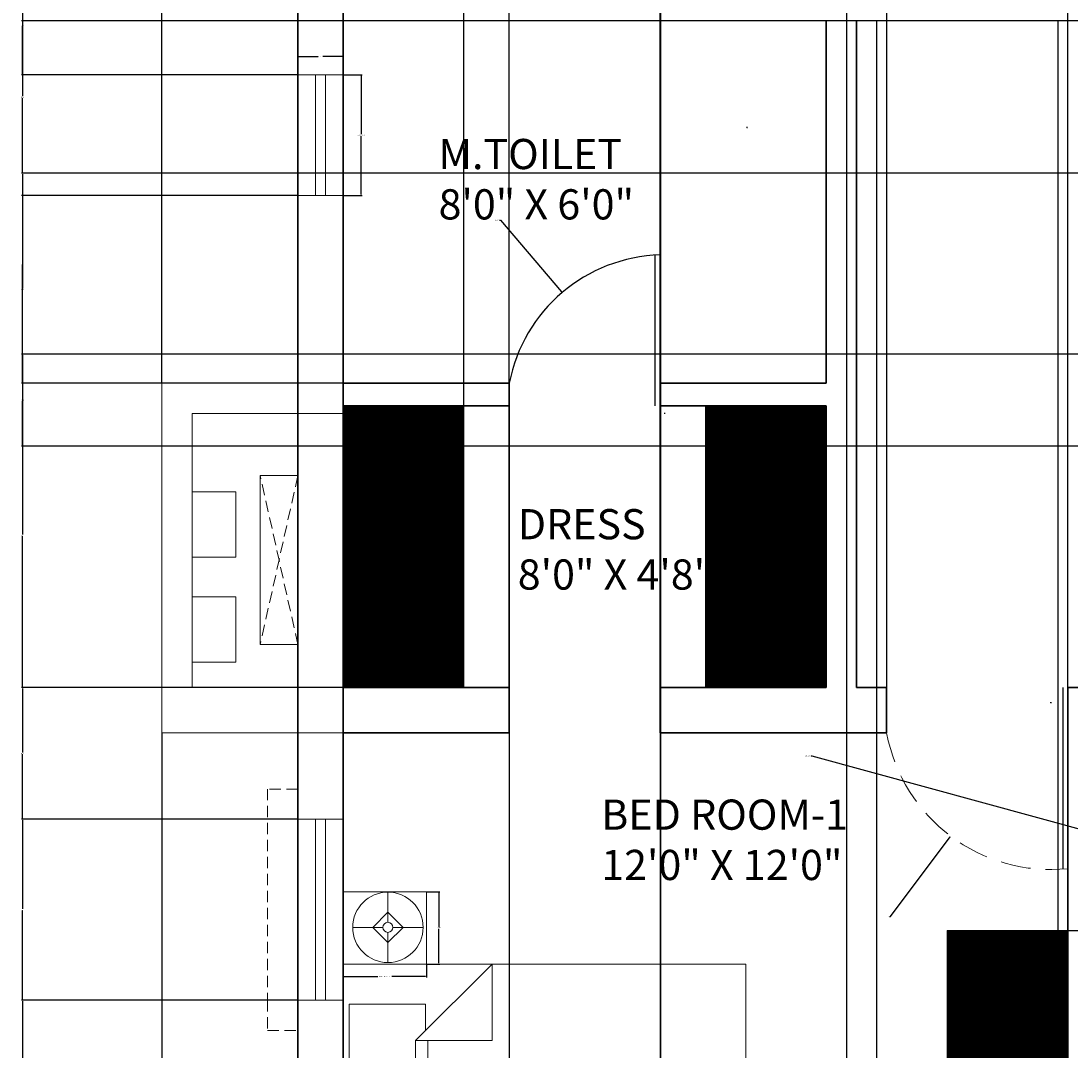
# Model space of a CAD drawing. Units: inches. Extents: x 6662 to 7211, y 5077 to 5683.
# Tile 2 of 9: x 6662 to 6870, y 5260 to 5465. Entities that reach past the tile are written whole.
import ezdxf

# ---------------------------------------------------------------- set-up
doc = ezdxf.new("R2010")
doc.units = ezdxf.units.IN
doc.header["$LTSCALE"] = 3
doc.header["$MEASUREMENT"] = 0
doc.linetypes.add('HIDDEN', pattern=[0.375, 0.25, -0.125])
for name, color, linetype, lineweight in [('A-ANNO-DIMS', 2, 'Continuous', 18), ('A-AREA-IDEN', 7, 'Continuous', 18), ('A-DOOR', 4, 'Continuous', 25), ('A-DOOR-HIDN', 4, 'HIDDEN', 13), ('A-FLOR-CASE', 8, 'Continuous', 20), ('A-FLOR-CASE-PATT', 241, 'Continuous', 13), ('A-FLOR-PROJ', 7, 'Continuous', 18), ('A-FLOR-PROJ-HIDN', 7, 'HIDDEN', 13), ('A-FURN', 8, 'Continuous', 18), ('A-GLAZ', 4, 'Continuous', 18), ('A-GLAZ-OVHD', 4, 'HIDDEN', 13), ('A-WALL', 7, 'Continuous', 35)]:
    doc.layers.add(name, color=color, linetype=linetype, lineweight=lineweight)
doc.styles.get("Standard").update_dxf_attribs({"font": 'arial.ttf'})
doc.dimstyles.get("Standard").update_dxf_attribs({"dimtxt": 0.18, "dimasz": 0.18, "dimexe": 0.18, "dimexo": 0.0625, "dimgap": 0.09, "dimtad": 0, "dimtih": 1, "dimtoh": 1, "dimdec": 4, "dimzin": 0, "dimdsep": 46, "dimtxsty": 'Standard', "dimcen": 0.09, "dimadec": 0, "dimazin": 0, "dimtfac": 1, "dimtdec": 4, "dimtofl": 0, "dimtmove": 0, "dimatfit": 3, "dimfxl": 1, "dimtolj": 1, "dimtzin": 0, "dimarcsym": 0})

# ---------------------------------------------------------------- blocks, each defined once
blk = doc.blocks.new('Bed - Queen')
for p, q in [((0, -80.00003), (0, 0)), ((0, 0), (59.99999, 0)), ((59.99999, 0), (59.99999, -80.00003)), ((7.99999, -1.2), (28.79998, -1.2)), ((7.99999, -14.4), (7.99999, -1.2)), ((28.79998, -1.2), (28.79998, -14.4)), ((31.19999, -1.2), (51.99999, -1.2)), ((31.19999, -14.4), (31.19999, -1.2)), ((51.99999, -1.2), (51.99999, -16.4)), ((0, -14.4), (44.8, -14.4)), ((59.99999, -29.6), (44.8, -14.4)), ((44.8, -14.4), (44.8, -29.6)), ((51.99999, -16.4), (46.79936, -16.4)), ((44.8, -16.8), (0, -16.8)), ((44.8, -29.6), (59.99999, -29.6)), ((59.99999, -80.00003), (0, -80.00003))]:
    blk.add_line(p, q)
blk = doc.blocks.new('Lamp - Table')
for p, q in [((0, 7), (0, 1)), ((0, 3), (-3, 0)), ((3, 0), (0, 3)), ((-1, 0), (-7, 0)), ((-3, 0), (0, -3)), ((0, -3), (3, 0)), ((1, 0), (7, 0)), ((0, -1), (0, -7))]:
    blk.add_line(p, q)
for radius in [7, 1]:
    blk.add_circle((0, 0), radius)
blk = doc.blocks.new('WIN-VENT-24IN')
for p, q in [((0, 0), (0, 9)), ((24, 0), (24, 9)), ((0, 5.5), (24, 5.5)), ((0, 3.5), (24, 3.5))]:
    blk.add_line(p, q)
blk = doc.blocks.new('BEDSIDE-TABLE')
blk.add_lwpolyline([(0, 14.35), (16.56, 14.35), (16.56, 0), (0, 0)], close=True)
blk = doc.blocks.new('*D18')
at = {"layer": 'A-ANNO-DIMS', "color": 0, "lineweight": -2, "ltscale": 3, "transparency": 16777216}
for p, q in [((6725.86, 5277.09), (6725.86, 5274.49)), ((6742.42, 5277.09), (6742.42, 5274.49)), ((6726.04, 5274.67), (6732.76, 5274.67)), ((6742.24, 5274.67), (6735.51, 5274.67))]:
    blk.add_line(p, q, dxfattribs=at)
at = {"layer": 'A-ANNO-DIMS', "color": 0, "ltscale": 3, "transparency": 16777216}
for points in [[(6726.04, 5274.7), (6726.04, 5274.64), (6725.86, 5274.67)], [(6742.24, 5274.7), (6742.24, 5274.64), (6742.42, 5274.67)]]:
    blk.add_solid(points, dxfattribs=at)
at = {"layer": 'Defpoints', "color": 0, "ltscale": 3, "transparency": 16777216}
for p in [(6725.86, 5277.15), (6742.42, 5277.15), (6742.42, 5274.67)]:
    blk.add_point(p, dxfattribs=at)
at = {"layer": 'A-ANNO-DIMS', "color": 0, "ltscale": 3, "transparency": 16777216, "insert": (6734.14, 5274.67), "char_height": 0.18, "attachment_point": 5}
blk.add_mtext('\\A1;NIGHTSTAND 17 TYP.', dxfattribs=at)
blk = doc.blocks.new('*D19')
at = {"layer": 'A-ANNO-DIMS', "color": 0, "lineweight": -2, "ltscale": 3, "transparency": 16777216}
for p, q in [((6742.48, 5291.51), (6745.08, 5291.51)), ((6744.9, 5291.33), (6744.9, 5284.51)), ((6744.9, 5277.33), (6744.9, 5284.15)), ((6742.48, 5277.15), (6745.08, 5277.15))]:
    blk.add_line(p, q, dxfattribs=at)
at = {"layer": 'A-ANNO-DIMS', "color": 0, "ltscale": 3, "transparency": 16777216}
for points in [[(6744.87, 5291.33), (6744.93, 5291.33), (6744.9, 5291.51)], [(6744.87, 5277.33), (6744.93, 5277.33), (6744.9, 5277.15)]]:
    blk.add_solid(points, dxfattribs=at)
at = {"layer": 'Defpoints', "color": 0, "ltscale": 3, "transparency": 16777216}
for p in [(6742.42, 5291.51), (6744.9, 5291.51), (6742.42, 5277.15)]:
    blk.add_point(p, dxfattribs=at)
at = {"layer": 'A-ANNO-DIMS', "color": 0, "ltscale": 3, "transparency": 16777216, "insert": (6744.9, 5284.33), "char_height": 0.18, "attachment_point": 5}
blk.add_mtext('\\A1;14 TYP.', dxfattribs=at)
blk = doc.blocks.new('*D26')
at = {"layer": 'A-ANNO-DIMS', "color": 0, "lineweight": -2, "ltscale": 3, "transparency": 16777216}
for p, q in [((6725.92, 5453.91), (6729.64, 5453.91)), ((6729.46, 5453.73), (6729.46, 5442.09)), ((6729.46, 5430.09), (6729.46, 5441.73)), ((6725.92, 5429.91), (6729.64, 5429.91))]:
    blk.add_line(p, q, dxfattribs=at)
at = {"layer": 'A-ANNO-DIMS', "color": 0, "ltscale": 3, "transparency": 16777216}
for points in [[(6729.43, 5453.73), (6729.49, 5453.73), (6729.46, 5453.91)], [(6729.43, 5430.09), (6729.49, 5430.09), (6729.46, 5429.91)]]:
    blk.add_solid(points, dxfattribs=at)
at = {"layer": 'Defpoints', "color": 0, "ltscale": 3, "transparency": 16777216}
for p in [(6725.86, 5453.91), (6725.86, 5429.91), (6729.46, 5429.91)]:
    blk.add_point(p, dxfattribs=at)
at = {"layer": 'A-ANNO-DIMS', "color": 0, "ltscale": 3, "transparency": 16777216, "insert": (6729.46, 5441.91), "char_height": 0.18, "attachment_point": 5}
blk.add_mtext('\\A1;VENT 24 TYP.', dxfattribs=at)
blk = doc.blocks.new('*D27')
at = {"layer": 'A-ANNO-DIMS', "color": 0, "lineweight": -2, "ltscale": 3, "transparency": 16777216}
for p, q in [((6716.86, 5453.97), (6716.86, 5457.69)), ((6717.04, 5457.51), (6720.9, 5457.51)), ((6725.68, 5457.51), (6721.82, 5457.51)), ((6725.86, 5453.97), (6725.86, 5457.69))]:
    blk.add_line(p, q, dxfattribs=at)
at = {"layer": 'A-ANNO-DIMS', "color": 0, "ltscale": 3, "transparency": 16777216}
for points in [[(6717.04, 5457.54), (6717.04, 5457.48), (6716.86, 5457.51)], [(6725.68, 5457.54), (6725.68, 5457.48), (6725.86, 5457.51)]]:
    blk.add_solid(points, dxfattribs=at)
at = {"layer": 'Defpoints', "color": 0, "ltscale": 3, "transparency": 16777216}
for p in [(6725.86, 5457.51), (6716.86, 5453.91), (6725.86, 5453.91)]:
    blk.add_point(p, dxfattribs=at)
at = {"layer": 'A-ANNO-DIMS', "color": 0, "ltscale": 3, "transparency": 16777216, "insert": (6721.36, 5457.51), "char_height": 0.18, "attachment_point": 5}
blk.add_mtext('\\A1;9 TYP.', dxfattribs=at)
blk = doc.blocks.new('*D40')
at = {"layer": 'A-ANNO-DIMS', "color": 0, "lineweight": -2, "ltscale": 3, "transparency": 16777216}
for p, q in [((7182.86, 5326.04), (7182.86, 5076.72)), ((6689.86, 5323.04), (6689.86, 5076.72)), ((6690.04, 5076.9), (6936.07, 5076.9)), ((7182.68, 5076.9), (6936.65, 5076.9))]:
    blk.add_line(p, q, dxfattribs=at)
at = {"layer": 'A-ANNO-DIMS', "color": 0, "ltscale": 3, "transparency": 16777216}
for points in [[(6690.04, 5076.93), (6690.04, 5076.87), (6689.86, 5076.9)], [(7182.68, 5076.93), (7182.68, 5076.87), (7182.86, 5076.9)]]:
    blk.add_solid(points, dxfattribs=at)
at = {"layer": 'Defpoints', "color": 0, "ltscale": 3, "transparency": 16777216}
for p in [(7182.86, 5326.1), (6689.86, 5323.1), (7182.86, 5076.9)]:
    blk.add_point(p, dxfattribs=at)
at = {"layer": 'A-ANNO-DIMS', "color": 0, "ltscale": 3, "transparency": 16777216, "insert": (6936.36, 5076.9), "char_height": 0.18, "attachment_point": 5}
blk.add_mtext('\\A1;493', dxfattribs=at)
blk = doc.blocks.new('*D42')
at = {"layer": 'A-ANNO-DIMS', "color": 0, "lineweight": -2, "ltscale": 3, "transparency": 16777216}
for p, q in [((6689.86, 5392.66), (6689.86, 5682.9)), ((6690.04, 5682.72), (6703.14, 5682.72)), ((6716.68, 5682.72), (6703.58, 5682.72)), ((6716.86, 5626.66), (6716.86, 5682.9))]:
    blk.add_line(p, q, dxfattribs=at)
at = {"layer": 'A-ANNO-DIMS', "color": 0, "ltscale": 3, "transparency": 16777216}
for points in [[(6690.04, 5682.75), (6690.04, 5682.69), (6689.86, 5682.72)], [(6716.68, 5682.75), (6716.68, 5682.69), (6716.86, 5682.72)]]:
    blk.add_solid(points, dxfattribs=at)
at = {"layer": 'Defpoints', "color": 0, "ltscale": 3, "transparency": 16777216}
for p in [(6716.86, 5682.72), (6716.86, 5626.6), (6689.86, 5392.6)]:
    blk.add_point(p, dxfattribs=at)
at = {"layer": 'A-ANNO-DIMS', "color": 0, "ltscale": 3, "transparency": 16777216, "insert": (6703.36, 5682.72), "char_height": 0.18, "attachment_point": 5}
blk.add_mtext('\\A1;27', dxfattribs=at)
blk = doc.blocks.new('*D54')
at = {"layer": 'A-ANNO-DIMS', "color": 0, "lineweight": -2, "ltscale": 3, "transparency": 16777216}
for p, q in [((6725.8, 5473.6), (6661.98, 5473.6)), ((6662.16, 5473.42), (6662.16, 5463.93)), ((6662.16, 5454.09), (6662.16, 5463.57)), ((6716.8, 5453.91), (6661.98, 5453.91))]:
    blk.add_line(p, q, dxfattribs=at)
at = {"layer": 'A-ANNO-DIMS', "color": 0, "ltscale": 3, "transparency": 16777216}
for points in [[(6662.13, 5473.42), (6662.19, 5473.42), (6662.16, 5473.6)], [(6662.13, 5454.09), (6662.19, 5454.09), (6662.16, 5453.91)]]:
    blk.add_solid(points, dxfattribs=at)
at = {"layer": 'Defpoints', "color": 0, "ltscale": 3, "transparency": 16777216}
for p in [(6662.16, 5473.6), (6725.86, 5473.6), (6716.86, 5453.91)]:
    blk.add_point(p, dxfattribs=at)
at = {"layer": 'A-ANNO-DIMS', "color": 0, "ltscale": 3, "transparency": 16777216, "insert": (6662.16, 5463.75), "char_height": 0.18, "attachment_point": 5}
blk.add_mtext('\\A1;19.69', dxfattribs=at)
blk = doc.blocks.new('*D55')
at = {"layer": 'A-ANNO-DIMS', "color": 0, "lineweight": -2, "ltscale": 3, "transparency": 16777216}
for p, q in [((6716.8, 5429.91), (6661.98, 5429.91)), ((6662.16, 5429.73), (6662.16, 5411.43)), ((6662.16, 5392.78), (6662.16, 5411.07)), ((6725.8, 5392.6), (6661.98, 5392.6))]:
    blk.add_line(p, q, dxfattribs=at)
at = {"layer": 'A-ANNO-DIMS', "color": 0, "ltscale": 3, "transparency": 16777216}
for points in [[(6662.13, 5429.73), (6662.19, 5429.73), (6662.16, 5429.91)], [(6662.13, 5392.78), (6662.19, 5392.78), (6662.16, 5392.6)]]:
    blk.add_solid(points, dxfattribs=at)
at = {"layer": 'Defpoints', "color": 0, "ltscale": 3, "transparency": 16777216}
for p in [(6716.86, 5429.91), (6662.16, 5392.6), (6725.86, 5392.6)]:
    blk.add_point(p, dxfattribs=at)
at = {"layer": 'A-ANNO-DIMS', "color": 0, "ltscale": 3, "transparency": 16777216, "insert": (6662.16, 5411.25), "char_height": 0.18, "attachment_point": 5}
blk.add_mtext('\\A1;37.31', dxfattribs=at)
blk = doc.blocks.new('*D56')
at = {"layer": 'A-ANNO-DIMS', "color": 0, "lineweight": -2, "ltscale": 3, "transparency": 16777216}
for p, q in [((6725.8, 5392.6), (6661.98, 5392.6)), ((6662.16, 5392.42), (6662.16, 5362.53)), ((6662.16, 5332.28), (6662.16, 5362.17)), ((6725.8, 5332.1), (6661.98, 5332.1))]:
    blk.add_line(p, q, dxfattribs=at)
at = {"layer": 'A-ANNO-DIMS', "color": 0, "ltscale": 3, "transparency": 16777216}
for points in [[(6662.13, 5392.42), (6662.19, 5392.42), (6662.16, 5392.6)], [(6662.13, 5332.28), (6662.19, 5332.28), (6662.16, 5332.1)]]:
    blk.add_solid(points, dxfattribs=at)
at = {"layer": 'Defpoints', "color": 0, "ltscale": 3, "transparency": 16777216}
for p in [(6725.86, 5392.6), (6662.16, 5332.1), (6725.86, 5332.1)]:
    blk.add_point(p, dxfattribs=at)
at = {"layer": 'A-ANNO-DIMS', "color": 0, "ltscale": 3, "transparency": 16777216, "insert": (6662.16, 5362.35), "char_height": 0.18, "attachment_point": 5}
blk.add_mtext('\\A1;60.5', dxfattribs=at)
blk = doc.blocks.new('*D57')
at = {"layer": 'A-ANNO-DIMS', "color": 0, "lineweight": -2, "ltscale": 3, "transparency": 16777216}
for p, q in [((6725.8, 5332.1), (6661.98, 5332.1)), ((6662.16, 5331.92), (6662.16, 5319.2)), ((6662.16, 5306.12), (6662.16, 5318.84)), ((6716.8, 5305.94), (6661.98, 5305.94))]:
    blk.add_line(p, q, dxfattribs=at)
at = {"layer": 'A-ANNO-DIMS', "color": 0, "ltscale": 3, "transparency": 16777216}
for points in [[(6662.13, 5331.92), (6662.19, 5331.92), (6662.16, 5332.1)], [(6662.13, 5306.12), (6662.19, 5306.12), (6662.16, 5305.94)]]:
    blk.add_solid(points, dxfattribs=at)
at = {"layer": 'Defpoints', "color": 0, "ltscale": 3, "transparency": 16777216}
for p in [(6725.86, 5332.1), (6662.16, 5305.94), (6716.86, 5305.94)]:
    blk.add_point(p, dxfattribs=at)
at = {"layer": 'A-ANNO-DIMS', "color": 0, "ltscale": 3, "transparency": 16777216, "insert": (6662.16, 5319.02), "char_height": 0.18, "attachment_point": 5}
blk.add_mtext('\\A1;26.16', dxfattribs=at)
blk = doc.blocks.new('*D58')
at = {"layer": 'A-ANNO-DIMS', "color": 0, "lineweight": -2, "ltscale": 3, "transparency": 16777216}
for p, q in [((6716.8, 5305.94), (6661.98, 5305.94)), ((6662.16, 5305.76), (6662.16, 5288.12)), ((6662.16, 5270.12), (6662.16, 5287.76)), ((6716.8, 5269.94), (6661.98, 5269.94))]:
    blk.add_line(p, q, dxfattribs=at)
at = {"layer": 'A-ANNO-DIMS', "color": 0, "ltscale": 3, "transparency": 16777216}
for points in [[(6662.13, 5305.76), (6662.19, 5305.76), (6662.16, 5305.94)], [(6662.13, 5270.12), (6662.19, 5270.12), (6662.16, 5269.94)]]:
    blk.add_solid(points, dxfattribs=at)
at = {"layer": 'Defpoints', "color": 0, "ltscale": 3, "transparency": 16777216}
for p in [(6716.86, 5305.94), (6662.16, 5269.94), (6716.86, 5269.94)]:
    blk.add_point(p, dxfattribs=at)
at = {"layer": 'A-ANNO-DIMS', "color": 0, "ltscale": 3, "transparency": 16777216, "insert": (6662.16, 5287.94), "char_height": 0.18, "attachment_point": 5}
blk.add_mtext('\\A1;36', dxfattribs=at)
blk = doc.blocks.new('*D59')
at = {"layer": 'A-ANNO-DIMS', "color": 0, "lineweight": -2, "ltscale": 3, "transparency": 16777216}
for p, q in [((6716.8, 5269.94), (6661.98, 5269.94)), ((6662.16, 5269.76), (6662.16, 5220.2)), ((6662.16, 5170.28), (6662.16, 5219.84)), ((6716.8, 5170.1), (6661.98, 5170.1))]:
    blk.add_line(p, q, dxfattribs=at)
at = {"layer": 'A-ANNO-DIMS', "color": 0, "ltscale": 3, "transparency": 16777216}
for points in [[(6662.13, 5269.76), (6662.19, 5269.76), (6662.16, 5269.94)], [(6662.13, 5170.28), (6662.19, 5170.28), (6662.16, 5170.1)]]:
    blk.add_solid(points, dxfattribs=at)
at = {"layer": 'Defpoints', "color": 0, "ltscale": 3, "transparency": 16777216}
for p in [(6716.86, 5269.94), (6662.16, 5170.1), (6716.86, 5170.1)]:
    blk.add_point(p, dxfattribs=at)
at = {"layer": 'A-ANNO-DIMS', "color": 0, "ltscale": 3, "transparency": 16777216, "insert": (6662.16, 5220.02), "char_height": 0.18, "attachment_point": 5}
blk.add_mtext('\\A1;99.84', dxfattribs=at)
blk = doc.blocks.new('*D61')
at = {"layer": 'A-ANNO-DIMS', "color": 0, "lineweight": -2, "ltscale": 3, "transparency": 16777216}
for p, q in [((7167.8, 5434.35), (6661.98, 5434.35)), ((6662.16, 5434.17), (6662.16, 5416.53)), ((6662.16, 5398.53), (6662.16, 5416.17)), ((7167.8, 5398.35), (6661.98, 5398.35))]:
    blk.add_line(p, q, dxfattribs=at)
at = {"layer": 'A-ANNO-DIMS', "color": 0, "ltscale": 3, "transparency": 16777216}
for points in [[(6662.13, 5434.17), (6662.19, 5434.17), (6662.16, 5434.35)], [(6662.13, 5398.53), (6662.19, 5398.53), (6662.16, 5398.35)]]:
    blk.add_solid(points, dxfattribs=at)
at = {"layer": 'Defpoints', "color": 0, "ltscale": 3, "transparency": 16777216}
for p in [(6662.16, 5434.35), (7167.86, 5434.35), (7167.86, 5398.35)]:
    blk.add_point(p, dxfattribs=at)
at = {"layer": 'A-ANNO-DIMS', "color": 0, "ltscale": 3, "transparency": 16777216, "insert": (6662.16, 5416.35), "char_height": 0.18, "attachment_point": 5}
blk.add_mtext('\\A1;36', dxfattribs=at)
blk = doc.blocks.new('*D62')
at = {"layer": 'A-ANNO-DIMS', "color": 0, "lineweight": -2, "ltscale": 3, "transparency": 16777216}
for p, q in [((6758.86, 5388.04), (6758.86, 5076.72)), ((6788.86, 5388.04), (6788.86, 5076.72)), ((6759.04, 5076.9), (6773.64, 5076.9)), ((6788.68, 5076.9), (6774.08, 5076.9))]:
    blk.add_line(p, q, dxfattribs=at)
at = {"layer": 'A-ANNO-DIMS', "color": 0, "ltscale": 3, "transparency": 16777216}
for points in [[(6759.04, 5076.93), (6759.04, 5076.87), (6758.86, 5076.9)], [(6788.68, 5076.93), (6788.68, 5076.87), (6788.86, 5076.9)]]:
    blk.add_solid(points, dxfattribs=at)
at = {"layer": 'Defpoints', "color": 0, "ltscale": 3, "transparency": 16777216}
for p in [(6758.86, 5388.1), (6788.86, 5388.1), (6788.86, 5076.9)]:
    blk.add_point(p, dxfattribs=at)
at = {"layer": 'A-ANNO-DIMS', "color": 0, "ltscale": 3, "transparency": 16777216, "insert": (6773.86, 5076.9), "char_height": 0.18, "attachment_point": 5}
blk.add_mtext('\\A1;30', dxfattribs=at)
blk = doc.blocks.new('*D63')
at = {"layer": 'A-ANNO-DIMS', "color": 0, "lineweight": -2, "ltscale": 3, "transparency": 16777216}
for p, q in [((6758.86, 5332.16), (6758.86, 5682.9)), ((6759.04, 5682.72), (6773.64, 5682.72)), ((6788.68, 5682.72), (6774.08, 5682.72)), ((6788.86, 5332.16), (6788.86, 5682.9))]:
    blk.add_line(p, q, dxfattribs=at)
at = {"layer": 'A-ANNO-DIMS', "color": 0, "ltscale": 3, "transparency": 16777216}
for points in [[(6759.04, 5682.75), (6759.04, 5682.69), (6758.86, 5682.72)], [(6788.68, 5682.75), (6788.68, 5682.69), (6788.86, 5682.72)]]:
    blk.add_solid(points, dxfattribs=at)
at = {"layer": 'Defpoints', "color": 0, "ltscale": 3, "transparency": 16777216}
for p in [(6788.86, 5682.72), (6758.86, 5332.1), (6788.86, 5332.1)]:
    blk.add_point(p, dxfattribs=at)
at = {"layer": 'A-ANNO-DIMS', "color": 0, "ltscale": 3, "transparency": 16777216, "insert": (6773.86, 5682.72), "char_height": 0.18, "attachment_point": 5}
blk.add_mtext('\\A1;30', dxfattribs=at)
blk = doc.blocks.new('*D64')
at = {"layer": 'A-ANNO-DIMS', "color": 0, "lineweight": -2, "ltscale": 3, "transparency": 16777216}
for p, q in [((6833.86, 5332.16), (6833.86, 5682.9)), ((6834.04, 5682.72), (6851.64, 5682.72)), ((6869.68, 5682.72), (6852.08, 5682.72)), ((6869.86, 5332.16), (6869.86, 5682.9))]:
    blk.add_line(p, q, dxfattribs=at)
at = {"layer": 'A-ANNO-DIMS', "color": 0, "ltscale": 3, "transparency": 16777216}
for points in [[(6834.04, 5682.75), (6834.04, 5682.69), (6833.86, 5682.72)], [(6869.68, 5682.75), (6869.68, 5682.69), (6869.86, 5682.72)]]:
    blk.add_solid(points, dxfattribs=at)
at = {"layer": 'Defpoints', "color": 0, "ltscale": 3, "transparency": 16777216}
for p in [(6869.86, 5682.72), (6833.86, 5332.1), (6869.86, 5332.1)]:
    blk.add_point(p, dxfattribs=at)
at = {"layer": 'A-ANNO-DIMS', "color": 0, "ltscale": 3, "transparency": 16777216, "insert": (6851.86, 5682.72), "char_height": 0.18, "attachment_point": 5}
blk.add_mtext('\\A1;36', dxfattribs=at)
blk = doc.blocks.new('*D65')
at = {"layer": 'A-ANNO-DIMS', "color": 0, "lineweight": -2, "ltscale": 3, "transparency": 16777216}
for p, q in [((6831.86, 5464.54), (6831.86, 5076.72)), ((6867.86, 5464.54), (6867.86, 5076.72)), ((6832.04, 5076.9), (6849.64, 5076.9)), ((6867.68, 5076.9), (6850.08, 5076.9))]:
    blk.add_line(p, q, dxfattribs=at)
at = {"layer": 'A-ANNO-DIMS', "color": 0, "ltscale": 3, "transparency": 16777216}
for points in [[(6832.04, 5076.93), (6832.04, 5076.87), (6831.86, 5076.9)], [(6867.68, 5076.93), (6867.68, 5076.87), (6867.86, 5076.9)]]:
    blk.add_solid(points, dxfattribs=at)
at = {"layer": 'Defpoints', "color": 0, "ltscale": 3, "transparency": 16777216}
for p in [(6831.86, 5464.6), (6867.86, 5464.6), (6867.86, 5076.9)]:
    blk.add_point(p, dxfattribs=at)
at = {"layer": 'A-ANNO-DIMS', "color": 0, "ltscale": 3, "transparency": 16777216, "insert": (6849.86, 5076.9), "char_height": 0.18, "attachment_point": 5}
blk.add_mtext('\\A1;36', dxfattribs=at)
blk = doc.blocks.new('*D73')
at = {"layer": 'A-ANNO-DIMS', "color": 0, "lineweight": -2, "ltscale": 3, "transparency": 16777216}
for p, q in [((6725.86, 5179.16), (6725.86, 5682.9)), ((6726.04, 5682.72), (6757.03, 5682.72)), ((6788.79, 5682.72), (6757.79, 5682.72)), ((6788.97, 5179.16), (6788.97, 5682.9))]:
    blk.add_line(p, q, dxfattribs=at)
at = {"layer": 'A-ANNO-DIMS', "color": 0, "ltscale": 3, "transparency": 16777216}
for points in [[(6726.04, 5682.75), (6726.04, 5682.69), (6725.86, 5682.72)], [(6788.79, 5682.75), (6788.79, 5682.69), (6788.97, 5682.72)]]:
    blk.add_solid(points, dxfattribs=at)
at = {"layer": 'Defpoints', "color": 0, "ltscale": 3, "transparency": 16777216}
for p in [(6788.97, 5682.72), (6725.86, 5179.1), (6788.97, 5179.1)]:
    blk.add_point(p, dxfattribs=at)
at = {"layer": 'A-ANNO-DIMS', "color": 0, "ltscale": 3, "transparency": 16777216, "insert": (6757.41, 5682.72), "char_height": 0.18, "attachment_point": 5}
blk.add_mtext('\\A1;63.11', dxfattribs=at)
blk = doc.blocks.new('*D76')
at = {"layer": 'A-ANNO-DIMS', "color": 0, "lineweight": -2, "ltscale": 3, "transparency": 16777216}
for p, q in [((7167.8, 5464.6), (6661.98, 5464.6)), ((6662.16, 5464.42), (6662.16, 5449.65)), ((6662.16, 5434.53), (6662.16, 5449.29)), ((7167.8, 5434.35), (6661.98, 5434.35))]:
    blk.add_line(p, q, dxfattribs=at)
at = {"layer": 'A-ANNO-DIMS', "color": 0, "ltscale": 3, "transparency": 16777216}
for points in [[(6662.13, 5464.42), (6662.19, 5464.42), (6662.16, 5464.6)], [(6662.13, 5434.53), (6662.19, 5434.53), (6662.16, 5434.35)]]:
    blk.add_solid(points, dxfattribs=at)
at = {"layer": 'Defpoints', "color": 0, "ltscale": 3, "transparency": 16777216}
for p in [(7167.86, 5464.6), (6662.16, 5434.35), (7167.86, 5434.35)]:
    blk.add_point(p, dxfattribs=at)
at = {"layer": 'A-ANNO-DIMS', "color": 0, "ltscale": 3, "transparency": 16777216, "insert": (6662.16, 5449.47), "char_height": 0.18, "attachment_point": 5}
blk.add_mtext('\\A1;30.25', dxfattribs=at)
blk = doc.blocks.new('*D77')
at = {"layer": 'A-ANNO-DIMS', "color": 0, "lineweight": -2, "ltscale": 3, "transparency": 16777216}
for p, q in [((7167.8, 5398.35), (6661.98, 5398.35)), ((6662.16, 5398.17), (6662.16, 5389.4)), ((6662.16, 5380.28), (6662.16, 5389.04)), ((7167.8, 5380.1), (6661.98, 5380.1))]:
    blk.add_line(p, q, dxfattribs=at)
at = {"layer": 'A-ANNO-DIMS', "color": 0, "ltscale": 3, "transparency": 16777216}
for points in [[(6662.13, 5398.17), (6662.19, 5398.17), (6662.16, 5398.35)], [(6662.13, 5380.28), (6662.19, 5380.28), (6662.16, 5380.1)]]:
    blk.add_solid(points, dxfattribs=at)
at = {"layer": 'Defpoints', "color": 0, "ltscale": 3, "transparency": 16777216}
for p in [(7167.86, 5398.35), (6662.16, 5380.1), (7167.86, 5380.1)]:
    blk.add_point(p, dxfattribs=at)
at = {"layer": 'A-ANNO-DIMS', "color": 0, "ltscale": 3, "transparency": 16777216, "insert": (6662.16, 5389.22), "char_height": 0.18, "attachment_point": 5}
blk.add_mtext('\\A1;18.25', dxfattribs=at)
blk = doc.blocks.new('*D79')
at = {"layer": 'A-ANNO-DIMS', "color": 0, "lineweight": -2, "ltscale": 3, "transparency": 16777216}
for p, q in [((6725.86, 5473.54), (6725.86, 5076.72)), ((6825.9, 5473.54), (6825.9, 5076.72)), ((6726.04, 5076.9), (6775.42, 5076.9)), ((6825.72, 5076.9), (6776.33, 5076.9))]:
    blk.add_line(p, q, dxfattribs=at)
at = {"layer": 'A-ANNO-DIMS', "color": 0, "ltscale": 3, "transparency": 16777216}
for points in [[(6726.04, 5076.93), (6726.04, 5076.87), (6725.86, 5076.9)], [(6825.72, 5076.93), (6825.72, 5076.87), (6825.9, 5076.9)]]:
    blk.add_solid(points, dxfattribs=at)
at = {"layer": 'Defpoints', "color": 0, "ltscale": 3, "transparency": 16777216}
for p in [(6725.86, 5473.6), (6825.9, 5473.6), (6825.9, 5076.9)]:
    blk.add_point(p, dxfattribs=at)
at = {"layer": 'A-ANNO-DIMS', "color": 0, "ltscale": 3, "transparency": 16777216, "insert": (6775.88, 5076.9), "char_height": 0.18, "attachment_point": 5}
blk.add_mtext('\\A1;100.04', dxfattribs=at)
blk = doc.blocks.new('*D83')
at = {"layer": 'A-ANNO-DIMS', "color": 0, "lineweight": -2, "ltscale": 3, "transparency": 16777216}
for p, q in [((6845.92, 5283.8), (7210.74, 5283.8)), ((7210.56, 5283.62), (7210.56, 5231.63)), ((7210.56, 5179.28), (7210.56, 5231.27)), ((6845.92, 5179.1), (7210.74, 5179.1))]:
    blk.add_line(p, q, dxfattribs=at)
at = {"layer": 'A-ANNO-DIMS', "color": 0, "ltscale": 3, "transparency": 16777216}
for points in [[(7210.53, 5283.62), (7210.59, 5283.62), (7210.56, 5283.8)], [(7210.53, 5179.28), (7210.59, 5179.28), (7210.56, 5179.1)]]:
    blk.add_solid(points, dxfattribs=at)
at = {"layer": 'Defpoints', "color": 0, "ltscale": 3, "transparency": 16777216}
for p in [(6845.86, 5283.8), (7210.56, 5283.8), (6845.86, 5179.1)]:
    blk.add_point(p, dxfattribs=at)
at = {"layer": 'A-ANNO-DIMS', "color": 0, "ltscale": 3, "transparency": 16777216, "insert": (7210.56, 5231.45), "char_height": 0.18, "attachment_point": 5}
blk.add_mtext('\\A1;104.7', dxfattribs=at)
blk = doc.blocks.new('*D84')
at = {"layer": 'A-ANNO-DIMS', "color": 0, "lineweight": -2, "ltscale": 3, "transparency": 16777216}
for p, q in [((6725.86, 5388.16), (6725.86, 5682.9)), ((6726.04, 5682.72), (6737.64, 5682.72)), ((6749.68, 5682.72), (6738.08, 5682.72)), ((6749.86, 5388.16), (6749.86, 5682.9))]:
    blk.add_line(p, q, dxfattribs=at)
at = {"layer": 'A-ANNO-DIMS', "color": 0, "ltscale": 3, "transparency": 16777216}
for points in [[(6726.04, 5682.75), (6726.04, 5682.69), (6725.86, 5682.72)], [(6749.68, 5682.75), (6749.68, 5682.69), (6749.86, 5682.72)]]:
    blk.add_solid(points, dxfattribs=at)
at = {"layer": 'Defpoints', "color": 0, "ltscale": 3, "transparency": 16777216}
for p in [(6725.86, 5682.72), (6725.86, 5388.1), (6749.86, 5388.1)]:
    blk.add_point(p, dxfattribs=at)
at = {"layer": 'A-ANNO-DIMS', "color": 0, "ltscale": 3, "transparency": 16777216, "insert": (6737.86, 5682.72), "char_height": 0.18, "attachment_point": 5}
blk.add_mtext('\\A1;24', dxfattribs=at)
blk = doc.blocks.new('*D91')
at = {"layer": 'A-ANNO-DIMS', "color": 0, "lineweight": -2, "ltscale": 3, "transparency": 16777216}
for p, q in [((6866.42, 5329.14), (6866.6, 5329.14)), ((6866.51, 5329.05), (6866.51, 5329.23)), ((6834.63, 5286.63), (6846.48, 5302.43)), ((6834.45, 5286.63), (6834.63, 5286.63))]:
    blk.add_line(p, q, dxfattribs=at)
at = {"layer": 'A-ANNO-DIMS', "color": 0, "ltscale": 3, "transparency": 16777216}
blk.add_solid([(6846.46, 5302.45), (6846.5, 5302.41), (6846.59, 5302.57)], dxfattribs=at)
at = {"layer": 'Defpoints', "color": 0, "ltscale": 3, "transparency": 16777216}
for p in [(6866.51, 5329.14), (6846.59, 5302.57)]:
    blk.add_point(p, dxfattribs=at)
at = {"layer": 'A-ANNO-DIMS', "color": 0, "ltscale": 3, "transparency": 16777216, "insert": (6833.99, 5286.63), "char_height": 0.18, "attachment_point": 5}
blk.add_mtext('\\A1;R33.21', dxfattribs=at)
blk = doc.blocks.new('*D92')
at = {"layer": 'A-ANNO-DIMS', "color": 0, "lineweight": -2, "ltscale": 3, "transparency": 16777216}
for p, q in [((6756.96, 5425.01), (6757.14, 5425.01)), ((6757.14, 5425.01), (6769.26, 5410.75)), ((6789.69, 5386.62), (6789.87, 5386.62)), ((6789.78, 5386.53), (6789.78, 5386.71))]:
    blk.add_line(p, q, dxfattribs=at)
at = {"layer": 'A-ANNO-DIMS', "color": 0, "ltscale": 3, "transparency": 16777216}
blk.add_solid([(6769.29, 5410.77), (6769.24, 5410.73), (6769.38, 5410.61)], dxfattribs=at)
at = {"layer": 'Defpoints', "color": 0, "ltscale": 3, "transparency": 16777216}
for p in [(6769.38, 5410.61), (6789.78, 5386.62)]:
    blk.add_point(p, dxfattribs=at)
at = {"layer": 'A-ANNO-DIMS', "color": 0, "ltscale": 3, "transparency": 16777216, "insert": (6756.48, 5425.01), "char_height": 0.18, "attachment_point": 5}
blk.add_mtext('\\A1;R31.49', dxfattribs=at)
blk = doc.blocks.new('*D100')
at = {"layer": 'A-ANNO-DIMS', "color": 0, "lineweight": -2, "ltscale": 3, "transparency": 16777216}
for p, q in [((6818.84, 5318.55), (6819.02, 5318.55)), ((6819.02, 5318.55), (6888.99, 5299.4)), ((7005.96, 5267.35), (7006.14, 5267.35)), ((7006.05, 5267.26), (7006.05, 5267.44))]:
    blk.add_line(p, q, dxfattribs=at)
at = {"layer": 'A-ANNO-DIMS', "color": 0, "ltscale": 3, "transparency": 16777216}
blk.add_solid([(6888.99, 5299.43), (6888.98, 5299.37), (6889.16, 5299.35)], dxfattribs=at)
at = {"layer": 'Defpoints', "color": 0, "ltscale": 3, "transparency": 16777216}
for p in [(6889.16, 5299.35), (7006.05, 5267.35)]:
    blk.add_point(p, dxfattribs=at)
at = {"layer": 'A-ANNO-DIMS', "color": 0, "ltscale": 3, "transparency": 16777216, "insert": (6818.17, 5318.55), "char_height": 0.18, "attachment_point": 5}
blk.add_mtext('\\A1;2X R121.2', dxfattribs=at)
blk = doc.blocks.new('*D102')
at = {"layer": 'A-ANNO-DIMS', "color": 0, "lineweight": -2, "ltscale": 3, "transparency": 16777216}
for p, q in [((6796.04, 5545.78), (6796.22, 5545.78)), ((6796.22, 5545.78), (6799.92, 5507.59)), ((6806.05, 5443.46), (6806.23, 5443.46)), ((6806.14, 5443.37), (6806.14, 5443.55))]:
    blk.add_line(p, q, dxfattribs=at)
at = {"layer": 'A-ANNO-DIMS', "color": 0, "ltscale": 3, "transparency": 16777216}
blk.add_solid([(6799.95, 5507.59), (6799.89, 5507.59), (6799.94, 5507.41)], dxfattribs=at)
at = {"layer": 'Defpoints', "color": 0, "ltscale": 3, "transparency": 16777216}
for p in [(6799.94, 5507.41), (6806.14, 5443.46)]:
    blk.add_point(p, dxfattribs=at)
at = {"layer": 'A-ANNO-DIMS', "color": 0, "ltscale": 3, "transparency": 16777216, "insert": (6795.36, 5545.78), "char_height": 0.18, "attachment_point": 5}
blk.add_mtext('\\A1;4X R64.25', dxfattribs=at)

msp = doc.modelspace()

# ---------------------------------------------------------------- hatches: boundary and pattern name
at = {"layer": 'A-FLOR-CASE-PATT'}
h = msp.add_hatch(dxfattribs=at)
h.set_pattern_fill('ANSI31', color=256)
h.paths.add_polyline_path([(6869.8579, 5283.7981), (6845.8579, 5283.7981), (6845.8579, 5229.4653), (6847.018, 5229.7817, -0.54116316), (6849.0925, 5228.1371), (6849.7129, 5228.234, -0.50821327), (6851.018, 5227.2817), (6851.018, 5226.7817), (6855.018, 5227.2817), (6855.018, 5225.7817), (6851.018, 5225.2817), (6851.018, 5217.7817), (6851.018, 5210.2817), (6855.018, 5209.7817), (6855.018, 5208.2817), (6851.018, 5208.7817), (6851.018, 5208.2817, -0.41421356), (6850.018, 5207.2817), (6849.0925, 5207.4263, -0.50580924), (6847.1872, 5205.7355), (6845.8579, 5206.0981), (6845.8579, 5179.0979), (6869.8579, 5179.0979)])
h.paths.add_polyline_path([(7167.8579, 5497.5979), (7143.8579, 5497.5979), (7078.3579, 5497.5979), (7078.3579, 5473.5979), (7163.8579, 5473.5979), (7167.8579, 5473.5979)])
h.paths.add_polyline_path([(6825.9016, 5497.5979), (6725.8579, 5497.5979), (6725.8579, 5473.5979), (6825.9016, 5473.5979)])
h.paths.add_polyline_path([(6796.6359, 5485.2095), (6797.1359, 5489.2095), (6806.1359, 5489.2095), (6815.1359, 5489.2095), (6815.6359, 5485.2095), (6814.1359, 5485.2095), (6813.6359, 5489.2095), (6806.1359, 5489.2095), (6798.6359, 5489.2095), (6798.1359, 5485.2095)], flags=16)
h = msp.add_hatch(dxfattribs=at)
h.set_pattern_fill('ANSI31', color=256)
h.paths.add_polyline_path([(6749.8579, 5388.0979), (6725.8579, 5388.0979), (6725.8579, 5332.0979), (6749.8579, 5332.0979)])
h.paths.add_polyline_path([(6821.8579, 5388.0979), (6797.8579, 5388.0979), (6797.8579, 5332.0979), (6821.8579, 5332.0979)])

# ---------------------------------------------------------------- linework, layer by layer
at = {"layer": 'A-DOOR'}
for p, q in [((6787.8579, 5388.0979), (6787.8579, 5418.0979)), ((6788.8579, 5388.0979), (6788.8579, 5418.0979)), ((6868.8579, 5332.0979), (6868.8579, 5296.0979)), ((6869.8579, 5332.0979), (6869.8579, 5296.0979))]:
    msp.add_line(p, q, dxfattribs=at)
msp.add_arc((6789.7764, 5386.6202), 31.4911, 91.671524, 169.05755, dxfattribs=at)
at = {"layer": 'A-DOOR-HIDN', "ltscale": 8}
msp.add_arc((6866.5139, 5329.1393), 33.2102, 190.481241, 275.778964, dxfattribs=at)
at = {"layer": 'A-FLOR-CASE'}
for p, q in [((6749.8579, 5332.0979), (6749.8579, 5388.0979)), ((6797.8579, 5332.0979), (6797.8579, 5388.0979)), ((6845.8579, 5179.0979), (6845.8579, 5283.7981)), ((6869.8579, 5283.7981), (6845.8579, 5283.7981))]:
    msp.add_line(p, q, dxfattribs=at)
at = {"layer": 'A-FLOR-PROJ', "ltscale": 3}
for p, q in [((6689.8579, 5323.0979), (6689.8579, 5392.5979)), ((6689.8579, 5392.5979), (6725.8579, 5392.5979)), ((6695.8579, 5332.0979), (6695.8579, 5386.5979)), ((6695.8579, 5386.5979), (6725.8579, 5386.5979)), ((6725.8579, 5332.0979), (6695.8579, 5332.0979)), ((6725.8579, 5323.0979), (6689.8579, 5323.0979))]:
    msp.add_line(p, q, dxfattribs=at)
for points in [[(6716.8579, 5374.2286), (6709.3897, 5374.2286), (6709.3897, 5340.668), (6716.8579, 5340.668)], [(6695.8579, 5371.0093), (6704.5217, 5371.0093), (6704.5217, 5358.0194), (6695.8579, 5358.0194)], [(6695.8579, 5350.16), (6704.5217, 5350.16), (6704.5217, 5337.1701), (6695.8579, 5337.1701)]]:
    msp.add_lwpolyline(points, close=True, dxfattribs=at)
at = {"layer": 'A-FLOR-PROJ-HIDN', "ltscale": 3}
for p, q in [((6716.8579, 5374.2286), (6709.3897, 5340.668)), ((6716.8579, 5340.668), (6709.3897, 5374.2286))]:
    msp.add_line(p, q, dxfattribs=at)
at = {"layer": 'A-GLAZ'}
for p, q in [((6716.8579, 5305.94), (6725.8579, 5305.94)), ((6720.3579, 5305.94), (6720.3579, 5269.94)), ((6722.3579, 5305.94), (6722.3579, 5269.94)), ((6716.8579, 5269.94), (6725.8579, 5269.94))]:
    msp.add_line(p, q, dxfattribs=at)
at = {"layer": 'A-GLAZ-OVHD', "ltscale": 3}
for p, q in [((6716.8579, 5311.94), (6710.8579, 5311.94)), ((6710.8579, 5311.94), (6710.8579, 5269.94)), ((6716.8579, 5305.94), (6716.8579, 5311.94)), ((6710.8579, 5269.94), (6710.8579, 5263.94)), ((6710.8579, 5263.94), (6716.8579, 5263.94))]:
    msp.add_line(p, q, dxfattribs=at)
at = {"layer": 'A-WALL'}
for p, q in [((6716.8579, 5170.0979), (6716.8579, 5626.5979)), ((6725.8579, 5392.5979), (6725.8579, 5464.5979)), ((6821.8579, 5392.5979), (6821.8579, 5464.5979)), ((6827.8579, 5332.0979), (6827.8579, 5464.5979)), ((6758.8579, 5392.5979), (6725.8579, 5392.5979)), ((6758.8579, 5388.0979), (6758.8579, 5392.5979)), ((6821.8579, 5392.5979), (6788.8579, 5392.5979)), ((6788.8579, 5388.0979), (6788.8579, 5392.5979)), ((6725.8579, 5332.0979), (6725.8579, 5388.0979)), ((6758.8579, 5388.0979), (6725.8579, 5388.0979)), ((6821.8579, 5388.0979), (6788.8579, 5388.0979)), ((6821.8579, 5332.0979), (6821.8579, 5388.0979)), ((6758.8579, 5332.0979), (6725.8579, 5332.0979)), ((6758.8579, 5332.0979), (6758.8579, 5323.0979)), ((6821.8579, 5332.0979), (6788.8579, 5332.0979)), ((6788.8579, 5332.0979), (6788.8579, 5323.0979)), ((6833.8579, 5332.0979), (6827.8579, 5332.0979)), ((6833.8579, 5323.0979), (6833.8579, 5332.0979)), ((6878.8579, 5332.0979), (6869.8579, 5332.0979)), ((6869.8579, 5323.0979), (6869.8579, 5332.0979)), ((6725.8579, 5179.0979), (6725.8579, 5323.0979)), ((6758.8579, 5323.0979), (6725.8579, 5323.0979)), ((6833.8579, 5323.0979), (6788.8579, 5323.0979)), ((6869.8579, 5179.0979), (6869.8579, 5323.0979))]:
    msp.add_line(p, q, dxfattribs=at)

# ---------------------------------------------------------------- block references
at = {"layer": 'A-FURN'}
for name, p in [('BEDSIDE-TABLE', (6725.858, 5277.1531)), ('Lamp - Table', (6734.7584, 5284.4391))]:
    msp.add_blockref(name, p, dxfattribs=at)
at = {"layer": 'A-FURN', "rotation": 90}
msp.add_blockref('Bed - Queen', (6725.8579, 5217.1528), dxfattribs=at)
at = {"layer": 'A-GLAZ', "rotation": 270.0000000000048}
msp.add_blockref('WIN-VENT-24IN', (6716.8579, 5453.9079), dxfattribs=at)

# ---------------------------------------------------------------- texts
at = {"layer": 'A-AREA-IDEN', "ltscale": 3, "char_height": 6, "attachment_point": 1}
for s, insert in [('M.TOILET\\P8\'0" X 6\'0"', (6744.8231, 5441.1548)), ('DRESS\\P8\'0" X 4\'8"', (6760.5559, 5367.5747)), ('BED ROOM-1\\P12\'0" X 12\'0"', (6777.1445, 5309.8462))]:
    msp.add_mtext_dynamic_manual_height_columns(s, width=381.547883, gutter_width=1, heights=[0], dxfattribs=dict(at, insert=insert))

# ---------------------------------------------------------------- dimensions: what is measured, and where the dimension line sits
at = {"layer": 'A-ANNO-DIMS', "ltscale": 3}
for base, p1, p2, override, picture, middle in [((6716.8579, 5682.7209), (6689.8579, 5392.5979), (6716.8579, 5626.5979), {"dimdec": 0, "dimlfac": 1, "dimrnd": 0, "dimzin": 0, "dimdsep": 46, "dimlunit": 2}, '*D42', (6703.3579, 5682.7209)), ((6788.9657, 5682.7209), (6725.8579, 5179.0979), (6788.9657, 5179.0979), {"dimdec": 2, "dimlfac": 1, "dimrnd": 0, "dimzin": 0, "dimdsep": 46, "dimlunit": 2}, '*D73', (6757.4118, 5682.7209)), ((6725.8579, 5682.7209), (6749.8579, 5388.0979), (6725.8579, 5388.0979), {"dimdec": 0, "dimlfac": 1, "dimrnd": 0, "dimzin": 0, "dimdsep": 46, "dimlunit": 2}, '*D84', (6737.8579, 5682.7209)), ((6788.8579, 5682.7209), (6758.8579, 5332.0979), (6788.8579, 5332.0979), {"dimdec": 0, "dimlfac": 1, "dimrnd": 0, "dimzin": 0, "dimdsep": 46, "dimlunit": 2}, '*D63', (6773.8579, 5682.7209)), ((6869.8579, 5682.7209), (6833.8579, 5332.0979), (6869.8579, 5332.0979), {"dimdec": 0, "dimlfac": 1, "dimrnd": 0, "dimzin": 0, "dimdsep": 46, "dimlunit": 2}, '*D64', (6851.8579, 5682.7209)), ((6825.9016, 5076.8979), (6725.8579, 5473.5979), (6825.9016, 5473.5979), {"dimdec": 2, "dimlfac": 1, "dimrnd": 0, "dimzin": 0, "dimdsep": 46, "dimlunit": 2}, '*D79', (6775.8797, 5076.8979)), ((6867.8579, 5076.8979), (6831.8579, 5464.5979), (6867.8579, 5464.5979), {"dimdec": 0, "dimlfac": 1, "dimrnd": 0, "dimzin": 0, "dimdsep": 46, "dimlunit": 2}, '*D65', (6849.8579, 5076.8979)), ((6788.8579, 5076.8979), (6758.8579, 5388.0979), (6788.8579, 5388.0979), {"dimdec": 0, "dimlfac": 1, "dimrnd": 0, "dimzin": 0, "dimdsep": 46, "dimlunit": 2}, '*D62', (6773.8579, 5076.8979)), ((7182.8579, 5076.8979), (6689.8579, 5323.0979), (7182.8579, 5326.0979), {"dimdec": 0, "dimlfac": 1, "dimrnd": 0, "dimzin": 0, "dimdsep": 46, "dimlunit": 2}, '*D40', (6936.3579, 5076.8979))]:
    dim = msp.add_linear_dim(base=base, p1=p1, p2=p2, dimstyle='Standard', override=override, dxfattribs=at)
    dim.commit()
    dim.dimension.update_dxf_attribs({"geometry": picture, "text_midpoint": middle})
for center, mpoint, text, override, picture, middle in [((6806.1359, 5443.4595), (6799.936, 5507.4097), '4X <>', {"dimdec": 2, "dimlfac": 1, "dimrnd": 0, "dimzin": 0, "dimdsep": 46, "dimlunit": 2}, '*D102', (6795.3586, 5545.7798)), ((7006.0547, 5267.3479), (6889.1593, 5299.3502), '2X <>', {"dimdec": 1, "dimlfac": 1, "dimrnd": 0, "dimzin": 0, "dimdsep": 46, "dimlunit": 2}, '*D100', (6818.1683, 5318.5515))]:
    dim = msp.add_radius_dim(center=center, mpoint=mpoint, text=text, dimstyle='Standard', override=override, dxfattribs=at)
    dim.commit()
    dim.dimension.update_dxf_attribs({"geometry": picture, "text_midpoint": middle, "dimtype": 164})
for base, p1, p2, override, picture, middle in [((6662.1579, 5473.5979), (6716.8579, 5453.908), (6725.8579, 5473.5979), {"dimdec": 2, "dimlfac": 1, "dimrnd": 0, "dimzin": 0, "dimdsep": 46, "dimlunit": 2}, '*D54', (6662.1579, 5463.753)), ((6662.1579, 5434.3479), (7167.8579, 5464.5979), (7167.8579, 5434.3479), {"dimdec": 2, "dimlfac": 1, "dimrnd": 0, "dimzin": 0, "dimdsep": 46, "dimlunit": 2}, '*D76', (6662.1579, 5449.4729)), ((6662.1579, 5434.3479), (7167.8579, 5398.3479), (7167.8579, 5434.3479), {"dimdec": 0, "dimlfac": 1, "dimrnd": 0, "dimzin": 0, "dimdsep": 46, "dimlunit": 2}, '*D61', (6662.1579, 5416.3479)), ((6662.1579, 5392.5979), (6716.8579, 5429.908), (6725.8579, 5392.5979), {"dimdec": 2, "dimlfac": 1, "dimrnd": 0, "dimzin": 0, "dimdsep": 46, "dimlunit": 2}, '*D55', (6662.1579, 5411.253)), ((6662.1579, 5380.0979), (7167.8579, 5398.3479), (7167.8579, 5380.0979), {"dimdec": 2, "dimlfac": 1, "dimrnd": 0, "dimzin": 0, "dimdsep": 46, "dimlunit": 2}, '*D77', (6662.1579, 5389.2229)), ((6662.1579, 5332.0979), (6725.8579, 5392.5979), (6725.8579, 5332.0979), {"dimdec": 1, "dimlfac": 1, "dimrnd": 0, "dimzin": 0, "dimdsep": 46, "dimlunit": 2}, '*D56', (6662.1579, 5362.3479)), ((6662.1579, 5305.94), (6725.8579, 5332.0979), (6716.8579, 5305.94), {"dimdec": 2, "dimlfac": 1, "dimrnd": 0, "dimzin": 0, "dimdsep": 46, "dimlunit": 2}, '*D57', (6662.1579, 5319.019)), ((6662.1579, 5269.94), (6716.8579, 5305.94), (6716.8579, 5269.94), {"dimdec": 0, "dimlfac": 1, "dimrnd": 0, "dimzin": 0, "dimdsep": 46, "dimlunit": 2}, '*D58', (6662.1579, 5287.94)), ((7210.5579, 5283.7981), (6845.8579, 5179.0979), (6845.8579, 5283.7981), {"dimdec": 1, "dimlfac": 1, "dimrnd": 0, "dimzin": 0, "dimdsep": 46, "dimlunit": 2}, '*D83', (7210.5579, 5231.448)), ((6662.1579, 5170.0979), (6716.8579, 5269.94), (6716.8579, 5170.0979), {"dimdec": 2, "dimlfac": 1, "dimrnd": 0, "dimzin": 0, "dimdsep": 46, "dimlunit": 2}, '*D59', (6662.1579, 5220.019))]:
    dim = msp.add_linear_dim(base=base, p1=p1, p2=p2, angle=90, dimstyle='Standard', override=override, dxfattribs=at)
    dim.commit()
    dim.dimension.update_dxf_attribs({"geometry": picture, "text_midpoint": middle})
for base, p1, p2, angle, text, picture, middle in [((6725.8579, 5457.508), (6716.8579, 5453.908), (6725.8579, 5453.908), 0, '<> TYP.', '*D27', (6721.3579, 5457.508)), ((6729.4579, 5429.908), (6725.8579, 5453.908), (6725.8579, 5429.908), 270, 'VENT <> TYP.', '*D26', (6729.4579, 5441.908)), ((6744.9033, 5291.506), (6742.4191, 5277.1528), (6742.4191, 5291.506), 90, '<> TYP.', '*D19', (6744.9033, 5284.3294))]:
    dim = msp.add_linear_dim(base=base, p1=p1, p2=p2, angle=angle, text=text, dimstyle='Standard', override={"dimdec": 0, "dimlfac": 1, "dimrnd": 0, "dimzin": 0, "dimdsep": 46, "dimlunit": 2}, dxfattribs=at)
    dim.commit()
    dim.dimension.update_dxf_attribs({"geometry": picture, "text_midpoint": middle})
for center, mpoint, picture, middle in [((6789.7764, 5386.6202), (6769.3813, 5410.6146), '*D92', (6756.4842, 5425.0112)), ((6866.5139, 5329.1393), (6846.588, 5302.571), '*D91', (6833.99, 5286.6301))]:
    dim = msp.add_radius_dim(center=center, mpoint=mpoint, dimstyle='Standard', override={"dimdec": 2, "dimlfac": 1, "dimrnd": 0, "dimzin": 0, "dimdsep": 46, "dimlunit": 2}, dxfattribs=at)
    dim.commit()
    dim.dimension.update_dxf_attribs({"geometry": picture, "text_midpoint": middle, "dimtype": 164})
dim = msp.add_linear_dim(base=(6742.4191, 5274.6686), p1=(6725.8579, 5277.1528), p2=(6742.4191, 5277.1528), text='NIGHTSTAND <> TYP.', dimstyle='Standard', override={"dimdec": 0, "dimlfac": 1, "dimrnd": 0, "dimzin": 0, "dimdsep": 46, "dimlunit": 2}, dxfattribs=at)
dim.commit()
dim.dimension.update_dxf_attribs({"geometry": '*D18', "text_midpoint": (6734.1385, 5274.6686)})

doc.saveas('drawing.dxf')
